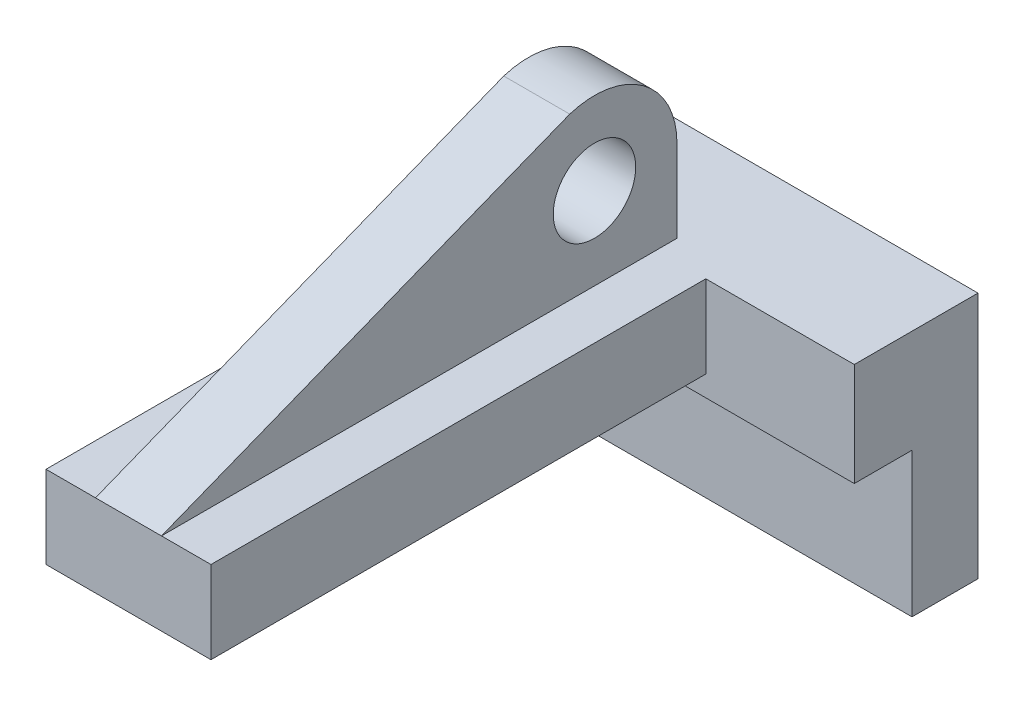
ISO-10303-21;
HEADER;
FILE_DESCRIPTION(('STEP AP214'),'2;1');
FILE_NAME('part.step','',(''),(''),'','','');
FILE_SCHEMA(('AUTOMOTIVE_DESIGN { 1 0 10303 214 1 1 1 1 }'));
ENDSEC;
DATA;
#1=APPLICATION_CONTEXT('core data for automotive mechanical design processes');
#2=APPLICATION_PROTOCOL_DEFINITION('international standard','automotive_design',2000,#1);
#3=PRODUCT_CONTEXT('',#1,'mechanical');
#4=PRODUCT('Part','Part','',(#3));
#5=PRODUCT_RELATED_PRODUCT_CATEGORY('part','',(#4));
#6=PRODUCT_DEFINITION_FORMATION('','',#4);
#7=PRODUCT_DEFINITION_CONTEXT('part definition',#1,'design');
#8=PRODUCT_DEFINITION('design','',#6,#7);
#9=PRODUCT_DEFINITION_SHAPE('','',#8);
#10=(LENGTH_UNIT() NAMED_UNIT(*) SI_UNIT(.MILLI.,.METRE.));
#11=(NAMED_UNIT(*) PLANE_ANGLE_UNIT() SI_UNIT($,.RADIAN.));
#12=(NAMED_UNIT(*) SI_UNIT($,.STERADIAN.) SOLID_ANGLE_UNIT());
#13=UNCERTAINTY_MEASURE_WITH_UNIT(LENGTH_MEASURE(1.E-05),#10,'distance_accuracy_value','');
#14=(GEOMETRIC_REPRESENTATION_CONTEXT(3) GLOBAL_UNCERTAINTY_ASSIGNED_CONTEXT((#13)) GLOBAL_UNIT_ASSIGNED_CONTEXT((#10,
#11,#12)) REPRESENTATION_CONTEXT('',''));
#15=CARTESIAN_POINT('',(0.,0.,0.));
#16=DIRECTION('',(0.,0.,1.));
#17=DIRECTION('',(1.,0.,0.));
#18=AXIS2_PLACEMENT_3D('',#15,#16,#17);
#19=CARTESIAN_POINT('',(0.,0.,25.));
#20=DIRECTION('',(0.,0.,1.));
#21=DIRECTION('',(1.,0.,0.));
#22=AXIS2_PLACEMENT_3D('',#19,#20,#21);
#23=PLANE('',#22);
#24=DIRECTION('',(0.,-1.,0.));
#25=VECTOR('',#24,1.);
#26=CARTESIAN_POINT('',(12.,0.,25.));
#27=LINE('',#26,#25);
#28=CARTESIAN_POINT('',(12.,80.,25.));
#29=VERTEX_POINT('',#28);
#30=CARTESIAN_POINT('',(12.,60.,25.));
#31=VERTEX_POINT('',#30);
#32=EDGE_CURVE('E158',#29,#31,#27,.T.);
#33=ORIENTED_EDGE('',*,*,#32,.F.);
#34=DIRECTION('',(1.,0.,0.));
#35=VECTOR('',#34,1.);
#36=CARTESIAN_POINT('',(0.,80.,25.));
#37=LINE('',#36,#35);
#38=CARTESIAN_POINT('',(28.,80.,25.));
#39=VERTEX_POINT('',#38);
#40=EDGE_CURVE('E61',#29,#39,#37,.T.);
#41=ORIENTED_EDGE('',*,*,#40,.T.);
#42=DIRECTION('',(0.,1.,0.));
#43=VECTOR('',#42,1.);
#44=CARTESIAN_POINT('',(28.,0.,25.));
#45=LINE('',#44,#43);
#46=CARTESIAN_POINT('',(28.,60.,25.));
#47=VERTEX_POINT('',#46);
#48=EDGE_CURVE('E161',#47,#39,#45,.T.);
#49=ORIENTED_EDGE('',*,*,#48,.F.);
#50=DIRECTION('',(1.,0.,0.));
#51=VECTOR('',#50,1.);
#52=CARTESIAN_POINT('',(0.,60.,25.));
#53=LINE('',#52,#51);
#54=EDGE_CURVE('E146',#31,#47,#53,.T.);
#55=ORIENTED_EDGE('',*,*,#54,.F.);
#56=EDGE_LOOP('',(#33,#41,#49,#55));
#57=FACE_BOUND('',#56,.T.);
#58=ADVANCED_FACE('F47',(#57),#23,.F.);
#59=CARTESIAN_POINT('',(0.,103.13948453494,40.7127457797623));
#60=DIRECTION('',(0.,-0.930155863944916,-0.367164906777439));
#61=DIRECTION('',(0.,0.367164906777439,-0.930155863944917));
#62=AXIS2_PLACEMENT_3D('',#59,#60,#61);
#63=PLANE('',#62);
#64=DIRECTION('',(0.,0.367164906777439,-0.930155863944917));
#65=VECTOR('',#64,1.);
#66=CARTESIAN_POINT('',(12.,103.13948453494,40.7127457797623));
#67=LINE('',#66,#65);
#68=CARTESIAN_POINT('',(12.,60.,150.));
#69=VERTEX_POINT('',#68);
#70=CARTESIAN_POINT('',(12.,99.0789287138878,50.9995399098919));
#71=VERTEX_POINT('',#70);
#72=EDGE_CURVE('E155',#69,#71,#67,.T.);
#73=ORIENTED_EDGE('',*,*,#72,.F.);
#74=DIRECTION('',(-1.,0.,0.));
#75=VECTOR('',#74,1.);
#76=CARTESIAN_POINT('',(40.,60.,150.));
#77=LINE('',#76,#75);
#78=CARTESIAN_POINT('',(28.,60.,150.));
#79=VERTEX_POINT('',#78);
#80=EDGE_CURVE('E192',#79,#69,#77,.T.);
#81=ORIENTED_EDGE('',*,*,#80,.F.);
#82=DIRECTION('',(0.,-0.367164906777439,0.930155863944917));
#83=VECTOR('',#82,1.);
#84=CARTESIAN_POINT('',(28.,103.13948453494,40.7127457797623));
#85=LINE('',#84,#83);
#86=CARTESIAN_POINT('',(28.,99.0789287138879,50.9995399098919));
#87=VERTEX_POINT('',#86);
#88=EDGE_CURVE('E523',#87,#79,#85,.T.);
#89=ORIENTED_EDGE('',*,*,#88,.F.);
#90=DIRECTION('',(1.,0.,0.));
#91=VECTOR('',#90,1.);
#92=CARTESIAN_POINT('',(0.,99.0789287138878,50.9995399098919));
#93=LINE('',#92,#91);
#94=EDGE_CURVE('E165',#71,#87,#93,.T.);
#95=ORIENTED_EDGE('',*,*,#94,.F.);
#96=EDGE_LOOP('',(#73,#81,#89,#95));
#97=FACE_BOUND('',#96,.T.);
#98=ADVANCED_FACE('F270',(#97),#63,.F.);
#99=CARTESIAN_POINT('',(0.,80.,45.));
#100=DIRECTION('',(1.,0.,0.));
#101=DIRECTION('',(0.,0.,-1.));
#102=AXIS2_PLACEMENT_3D('',#99,#100,#101);
#103=CYLINDRICAL_SURFACE('',#102,20.);
#104=ORIENTED_EDGE('',*,*,#40,.F.);
#105=CARTESIAN_POINT('',(12.,80.,45.));
#106=DIRECTION('',(-1.,0.,0.));
#107=DIRECTION('',(0.,0.,1.));
#108=AXIS2_PLACEMENT_3D('',#105,#106,#107);
#109=CIRCLE('',#108,20.);
#110=EDGE_CURVE('E156',#71,#29,#109,.T.);
#111=ORIENTED_EDGE('',*,*,#110,.F.);
#112=ORIENTED_EDGE('',*,*,#94,.T.);
#113=CARTESIAN_POINT('',(28.,80.,45.));
#114=DIRECTION('',(1.,0.,0.));
#115=DIRECTION('',(0.,0.,-1.));
#116=AXIS2_PLACEMENT_3D('',#113,#114,#115);
#117=CIRCLE('',#116,20.);
#118=EDGE_CURVE('E172',#39,#87,#117,.T.);
#119=ORIENTED_EDGE('',*,*,#118,.F.);
#120=EDGE_LOOP('',(#104,#111,#112,#119));
#121=FACE_BOUND('',#120,.T.);
#122=ADVANCED_FACE('F269',(#121),#103,.T.);
#123=CARTESIAN_POINT('',(0.,60.,16.));
#124=DIRECTION('',(1.,0.,0.));
#125=DIRECTION('',(0.,0.,-1.));
#126=AXIS2_PLACEMENT_3D('',#123,#124,#125);
#127=PLANE('',#126);
#128=DIRECTION('',(0.,1.,0.));
#129=VECTOR('',#128,1.);
#130=CARTESIAN_POINT('',(0.,60.,150.));
#131=LINE('',#130,#129);
#132=CARTESIAN_POINT('',(0.,40.,150.));
#133=VERTEX_POINT('',#132);
#134=CARTESIAN_POINT('',(0.,60.,150.));
#135=VERTEX_POINT('',#134);
#136=EDGE_CURVE('E168',#133,#135,#131,.T.);
#137=ORIENTED_EDGE('',*,*,#136,.T.);
#138=DIRECTION('',(0.,0.,-1.));
#139=VECTOR('',#138,1.);
#140=CARTESIAN_POINT('',(0.,60.,16.));
#141=LINE('',#140,#139);
#142=CARTESIAN_POINT('',(0.,60.,0.));
#143=VERTEX_POINT('',#142);
#144=EDGE_CURVE('E218',#135,#143,#141,.T.);
#145=ORIENTED_EDGE('',*,*,#144,.T.);
#146=DIRECTION('',(0.,-1.,0.));
#147=VECTOR('',#146,1.);
#148=CARTESIAN_POINT('',(0.,60.,0.));
#149=LINE('',#148,#147);
#150=CARTESIAN_POINT('',(0.,0.,0.));
#151=VERTEX_POINT('',#150);
#152=EDGE_CURVE('E208',#143,#151,#149,.T.);
#153=ORIENTED_EDGE('',*,*,#152,.T.);
#154=DIRECTION('',(0.,0.,-1.));
#155=VECTOR('',#154,1.);
#156=CARTESIAN_POINT('',(0.,0.,16.));
#157=LINE('',#156,#155);
#158=CARTESIAN_POINT('',(0.,0.,16.));
#159=VERTEX_POINT('',#158);
#160=EDGE_CURVE('E12',#159,#151,#157,.T.);
#161=ORIENTED_EDGE('',*,*,#160,.F.);
#162=DIRECTION('',(0.,-1.,0.));
#163=VECTOR('',#162,1.);
#164=CARTESIAN_POINT('',(0.,60.,16.));
#165=LINE('',#164,#163);
#166=CARTESIAN_POINT('',(0.,35.,16.));
#167=VERTEX_POINT('',#166);
#168=EDGE_CURVE('E212',#167,#159,#165,.T.);
#169=ORIENTED_EDGE('',*,*,#168,.F.);
#170=DIRECTION('',(0.,0.,-1.));
#171=VECTOR('',#170,1.);
#172=CARTESIAN_POINT('',(0.,35.,46.));
#173=LINE('',#172,#171);
#174=CARTESIAN_POINT('',(0.,35.,30.));
#175=VERTEX_POINT('',#174);
#176=EDGE_CURVE('E205',#175,#167,#173,.T.);
#177=ORIENTED_EDGE('',*,*,#176,.F.);
#178=DIRECTION('',(0.,-1.,0.));
#179=VECTOR('',#178,1.);
#180=CARTESIAN_POINT('',(0.,35.,30.));
#181=LINE('',#180,#179);
#182=CARTESIAN_POINT('',(0.,40.,30.));
#183=VERTEX_POINT('',#182);
#184=EDGE_CURVE('E188',#183,#175,#181,.T.);
#185=ORIENTED_EDGE('',*,*,#184,.F.);
#186=DIRECTION('',(0.,0.,1.));
#187=VECTOR('',#186,1.);
#188=CARTESIAN_POINT('',(0.,40.,150.));
#189=LINE('',#188,#187);
#190=EDGE_CURVE('E74',#183,#133,#189,.T.);
#191=ORIENTED_EDGE('',*,*,#190,.T.);
#192=EDGE_LOOP('',(#137,#145,#153,#161,#169,#177,#185,#191));
#193=FACE_BOUND('',#192,.T.);
#194=ADVANCED_FACE('F51',(#193),#127,.F.);
#195=CARTESIAN_POINT('',(0.,0.,16.));
#196=DIRECTION('',(0.,1.,0.));
#197=DIRECTION('',(0.,0.,1.));
#198=AXIS2_PLACEMENT_3D('',#195,#196,#197);
#199=PLANE('',#198);
#200=DIRECTION('',(1.,0.,0.));
#201=VECTOR('',#200,1.);
#202=CARTESIAN_POINT('',(0.,0.,0.));
#203=LINE('',#202,#201);
#204=CARTESIAN_POINT('',(76.,0.,0.));
#205=VERTEX_POINT('',#204);
#206=EDGE_CURVE('E224',#151,#205,#203,.T.);
#207=ORIENTED_EDGE('',*,*,#206,.T.);
#208=DIRECTION('',(0.,0.,-1.));
#209=VECTOR('',#208,1.);
#210=CARTESIAN_POINT('',(76.,0.,16.));
#211=LINE('',#210,#209);
#212=CARTESIAN_POINT('',(76.,0.,16.));
#213=VERTEX_POINT('',#212);
#214=EDGE_CURVE('E60',#213,#205,#211,.T.);
#215=ORIENTED_EDGE('',*,*,#214,.F.);
#216=DIRECTION('',(1.,0.,0.));
#217=VECTOR('',#216,1.);
#218=CARTESIAN_POINT('',(0.,0.,16.));
#219=LINE('',#218,#217);
#220=EDGE_CURVE('E214',#159,#213,#219,.T.);
#221=ORIENTED_EDGE('',*,*,#220,.F.);
#222=ORIENTED_EDGE('',*,*,#160,.T.);
#223=EDGE_LOOP('',(#207,#215,#221,#222));
#224=FACE_BOUND('',#223,.T.);
#225=ADVANCED_FACE('F256',(#224),#199,.F.);
#226=CARTESIAN_POINT('',(76.,0.,16.));
#227=DIRECTION('',(-1.,0.,0.));
#228=DIRECTION('',(0.,0.,1.));
#229=AXIS2_PLACEMENT_3D('',#226,#227,#228);
#230=PLANE('',#229);
#231=DIRECTION('',(0.,0.,-1.));
#232=VECTOR('',#231,1.);
#233=CARTESIAN_POINT('',(76.,60.,16.));
#234=LINE('',#233,#232);
#235=CARTESIAN_POINT('',(76.,60.,30.));
#236=VERTEX_POINT('',#235);
#237=CARTESIAN_POINT('',(76.,60.,0.));
#238=VERTEX_POINT('',#237);
#239=EDGE_CURVE('E229',#236,#238,#234,.T.);
#240=ORIENTED_EDGE('',*,*,#239,.F.);
#241=DIRECTION('',(0.,1.,0.));
#242=VECTOR('',#241,1.);
#243=CARTESIAN_POINT('',(76.,60.,30.));
#244=LINE('',#243,#242);
#245=CARTESIAN_POINT('',(76.,35.,30.));
#246=VERTEX_POINT('',#245);
#247=EDGE_CURVE('E199',#246,#236,#244,.T.);
#248=ORIENTED_EDGE('',*,*,#247,.F.);
#249=DIRECTION('',(0.,0.,-1.));
#250=VECTOR('',#249,1.);
#251=CARTESIAN_POINT('',(76.,35.,46.));
#252=LINE('',#251,#250);
#253=CARTESIAN_POINT('',(76.,35.,16.));
#254=VERTEX_POINT('',#253);
#255=EDGE_CURVE('E202',#246,#254,#252,.T.);
#256=ORIENTED_EDGE('',*,*,#255,.T.);
#257=DIRECTION('',(0.,1.,0.));
#258=VECTOR('',#257,1.);
#259=CARTESIAN_POINT('',(76.,0.,16.));
#260=LINE('',#259,#258);
#261=EDGE_CURVE('E216',#213,#254,#260,.T.);
#262=ORIENTED_EDGE('',*,*,#261,.F.);
#263=ORIENTED_EDGE('',*,*,#214,.T.);
#264=DIRECTION('',(0.,1.,0.));
#265=VECTOR('',#264,1.);
#266=CARTESIAN_POINT('',(76.,0.,0.));
#267=LINE('',#266,#265);
#268=EDGE_CURVE('E225',#205,#238,#267,.T.);
#269=ORIENTED_EDGE('',*,*,#268,.T.);
#270=EDGE_LOOP('',(#240,#248,#256,#262,#263,#269));
#271=FACE_BOUND('',#270,.T.);
#272=ADVANCED_FACE('F240',(#271),#230,.F.);
#273=CARTESIAN_POINT('',(76.,60.,16.));
#274=DIRECTION('',(0.,-1.,0.));
#275=DIRECTION('',(0.,0.,-1.));
#276=AXIS2_PLACEMENT_3D('',#273,#274,#275);
#277=PLANE('',#276);
#278=DIRECTION('',(0.,0.,-1.));
#279=VECTOR('',#278,1.);
#280=CARTESIAN_POINT('',(40.,60.,0.));
#281=LINE('',#280,#279);
#282=CARTESIAN_POINT('',(40.,60.,150.));
#283=VERTEX_POINT('',#282);
#284=CARTESIAN_POINT('',(40.,60.,30.));
#285=VERTEX_POINT('',#284);
#286=EDGE_CURVE('E167',#283,#285,#281,.T.);
#287=ORIENTED_EDGE('',*,*,#286,.T.);
#288=DIRECTION('',(-1.,0.,0.));
#289=VECTOR('',#288,1.);
#290=CARTESIAN_POINT('',(0.,60.,30.));
#291=LINE('',#290,#289);
#292=EDGE_CURVE('E200',#236,#285,#291,.T.);
#293=ORIENTED_EDGE('',*,*,#292,.F.);
#294=ORIENTED_EDGE('',*,*,#239,.T.);
#295=DIRECTION('',(-1.,0.,0.));
#296=VECTOR('',#295,1.);
#297=CARTESIAN_POINT('',(76.,60.,0.));
#298=LINE('',#297,#296);
#299=EDGE_CURVE('E211',#238,#143,#298,.T.);
#300=ORIENTED_EDGE('',*,*,#299,.T.);
#301=ORIENTED_EDGE('',*,*,#144,.F.);
#302=DIRECTION('',(-1.,0.,0.));
#303=VECTOR('',#302,1.);
#304=CARTESIAN_POINT('',(12.,60.,150.));
#305=LINE('',#304,#303);
#306=EDGE_CURVE('E152',#69,#135,#305,.T.);
#307=ORIENTED_EDGE('',*,*,#306,.F.);
#308=DIRECTION('',(0.,0.,1.));
#309=VECTOR('',#308,1.);
#310=CARTESIAN_POINT('',(12.,60.,0.));
#311=LINE('',#310,#309);
#312=EDGE_CURVE('E143',#31,#69,#311,.T.);
#313=ORIENTED_EDGE('',*,*,#312,.F.);
#314=ORIENTED_EDGE('',*,*,#54,.T.);
#315=DIRECTION('',(0.,0.,-1.));
#316=VECTOR('',#315,1.);
#317=CARTESIAN_POINT('',(28.,60.,0.));
#318=LINE('',#317,#316);
#319=EDGE_CURVE('E518',#79,#47,#318,.T.);
#320=ORIENTED_EDGE('',*,*,#319,.F.);
#321=EDGE_CURVE('E190',#283,#79,#77,.T.);
#322=ORIENTED_EDGE('',*,*,#321,.F.);
#323=EDGE_LOOP('',(#287,#293,#294,#300,#301,#307,#313,#314,#320,#322));
#324=FACE_BOUND('',#323,.T.);
#325=ADVANCED_FACE('F150',(#324),#277,.F.);
#326=CARTESIAN_POINT('',(0.,0.,16.));
#327=DIRECTION('',(0.,0.,1.));
#328=DIRECTION('',(1.,0.,0.));
#329=AXIS2_PLACEMENT_3D('',#326,#327,#328);
#330=PLANE('',#329);
#331=DIRECTION('',(1.,0.,0.));
#332=VECTOR('',#331,1.);
#333=CARTESIAN_POINT('',(0.,35.,16.));
#334=LINE('',#333,#332);
#335=EDGE_CURVE('E207',#167,#254,#334,.T.);
#336=ORIENTED_EDGE('',*,*,#335,.F.);
#337=ORIENTED_EDGE('',*,*,#168,.T.);
#338=ORIENTED_EDGE('',*,*,#220,.T.);
#339=ORIENTED_EDGE('',*,*,#261,.T.);
#340=EDGE_LOOP('',(#336,#337,#338,#339));
#341=FACE_BOUND('',#340,.T.);
#342=ADVANCED_FACE('F253',(#341),#330,.T.);
#343=CARTESIAN_POINT('',(0.,0.,0.));
#344=DIRECTION('',(0.,0.,1.));
#345=DIRECTION('',(1.,0.,0.));
#346=AXIS2_PLACEMENT_3D('',#343,#344,#345);
#347=PLANE('',#346);
#348=ORIENTED_EDGE('',*,*,#152,.F.);
#349=ORIENTED_EDGE('',*,*,#299,.F.);
#350=ORIENTED_EDGE('',*,*,#268,.F.);
#351=ORIENTED_EDGE('',*,*,#206,.F.);
#352=EDGE_LOOP('',(#348,#349,#350,#351));
#353=FACE_BOUND('',#352,.T.);
#354=ADVANCED_FACE('F243',(#353),#347,.F.);
#355=CARTESIAN_POINT('',(0.,35.,46.));
#356=DIRECTION('',(0.,-1.,0.));
#357=DIRECTION('',(0.,0.,-1.));
#358=AXIS2_PLACEMENT_3D('',#355,#356,#357);
#359=PLANE('',#358);
#360=DIRECTION('',(1.,0.,0.));
#361=VECTOR('',#360,1.);
#362=CARTESIAN_POINT('',(76.,35.,30.));
#363=LINE('',#362,#361);
#364=EDGE_CURVE('E196',#175,#246,#363,.T.);
#365=ORIENTED_EDGE('',*,*,#364,.F.);
#366=ORIENTED_EDGE('',*,*,#176,.T.);
#367=ORIENTED_EDGE('',*,*,#335,.T.);
#368=ORIENTED_EDGE('',*,*,#255,.F.);
#369=EDGE_LOOP('',(#365,#366,#367,#368));
#370=FACE_BOUND('',#369,.T.);
#371=ADVANCED_FACE('F249',(#370),#359,.T.);
#372=CARTESIAN_POINT('',(0.,0.,30.));
#373=DIRECTION('',(0.,0.,-1.));
#374=DIRECTION('',(-1.,0.,0.));
#375=AXIS2_PLACEMENT_3D('',#372,#373,#374);
#376=PLANE('',#375);
#377=ORIENTED_EDGE('',*,*,#292,.T.);
#378=DIRECTION('',(0.,-1.,0.));
#379=VECTOR('',#378,1.);
#380=CARTESIAN_POINT('',(40.,40.,30.));
#381=LINE('',#380,#379);
#382=CARTESIAN_POINT('',(40.,40.,30.));
#383=VERTEX_POINT('',#382);
#384=EDGE_CURVE('E174',#285,#383,#381,.T.);
#385=ORIENTED_EDGE('',*,*,#384,.T.);
#386=DIRECTION('',(-1.,0.,0.));
#387=VECTOR('',#386,1.);
#388=CARTESIAN_POINT('',(40.,40.,30.));
#389=LINE('',#388,#387);
#390=EDGE_CURVE('E182',#383,#183,#389,.T.);
#391=ORIENTED_EDGE('',*,*,#390,.T.);
#392=ORIENTED_EDGE('',*,*,#184,.T.);
#393=ORIENTED_EDGE('',*,*,#364,.T.);
#394=ORIENTED_EDGE('',*,*,#247,.T.);
#395=EDGE_LOOP('',(#377,#385,#391,#392,#393,#394));
#396=FACE_BOUND('',#395,.T.);
#397=ADVANCED_FACE('F289',(#396),#376,.F.);
#398=CARTESIAN_POINT('',(40.,60.,150.));
#399=DIRECTION('',(0.,0.,1.));
#400=DIRECTION('',(1.,0.,0.));
#401=AXIS2_PLACEMENT_3D('',#398,#399,#400);
#402=PLANE('',#401);
#403=ORIENTED_EDGE('',*,*,#136,.F.);
#404=DIRECTION('',(-1.,0.,0.));
#405=VECTOR('',#404,1.);
#406=CARTESIAN_POINT('',(40.,40.,150.));
#407=LINE('',#406,#405);
#408=CARTESIAN_POINT('',(40.,40.,150.));
#409=VERTEX_POINT('',#408);
#410=EDGE_CURVE('E195',#409,#133,#407,.T.);
#411=ORIENTED_EDGE('',*,*,#410,.F.);
#412=DIRECTION('',(0.,1.,0.));
#413=VECTOR('',#412,1.);
#414=CARTESIAN_POINT('',(40.,60.,150.));
#415=LINE('',#414,#413);
#416=EDGE_CURVE('E181',#409,#283,#415,.T.);
#417=ORIENTED_EDGE('',*,*,#416,.T.);
#418=ORIENTED_EDGE('',*,*,#321,.T.);
#419=ORIENTED_EDGE('',*,*,#80,.T.);
#420=ORIENTED_EDGE('',*,*,#306,.T.);
#421=EDGE_LOOP('',(#403,#411,#417,#418,#419,#420));
#422=FACE_BOUND('',#421,.T.);
#423=ADVANCED_FACE('F283',(#422),#402,.T.);
#424=CARTESIAN_POINT('',(40.,40.,150.));
#425=DIRECTION('',(0.,-1.,0.));
#426=DIRECTION('',(0.,0.,-1.));
#427=AXIS2_PLACEMENT_3D('',#424,#425,#426);
#428=PLANE('',#427);
#429=ORIENTED_EDGE('',*,*,#190,.F.);
#430=ORIENTED_EDGE('',*,*,#390,.F.);
#431=DIRECTION('',(0.,0.,1.));
#432=VECTOR('',#431,1.);
#433=CARTESIAN_POINT('',(40.,40.,150.));
#434=LINE('',#433,#432);
#435=EDGE_CURVE('E178',#383,#409,#434,.T.);
#436=ORIENTED_EDGE('',*,*,#435,.T.);
#437=ORIENTED_EDGE('',*,*,#410,.T.);
#438=EDGE_LOOP('',(#429,#430,#436,#437));
#439=FACE_BOUND('',#438,.T.);
#440=ADVANCED_FACE('F282',(#439),#428,.T.);
#441=CARTESIAN_POINT('',(40.,0.,0.));
#442=DIRECTION('',(1.,0.,0.));
#443=DIRECTION('',(0.,0.,-1.));
#444=AXIS2_PLACEMENT_3D('',#441,#442,#443);
#445=PLANE('',#444);
#446=ORIENTED_EDGE('',*,*,#286,.F.);
#447=ORIENTED_EDGE('',*,*,#416,.F.);
#448=ORIENTED_EDGE('',*,*,#435,.F.);
#449=ORIENTED_EDGE('',*,*,#384,.F.);
#450=EDGE_LOOP('',(#446,#447,#448,#449));
#451=FACE_BOUND('',#450,.T.);
#452=ADVANCED_FACE('F279',(#451),#445,.T.);
#453=CARTESIAN_POINT('',(28.,0.,0.));
#454=DIRECTION('',(1.,0.,0.));
#455=DIRECTION('',(0.,0.,-1.));
#456=AXIS2_PLACEMENT_3D('',#453,#454,#455);
#457=PLANE('',#456);
#458=CARTESIAN_POINT('',(28.,80.,45.));
#459=DIRECTION('',(1.,0.,0.));
#460=DIRECTION('',(0.,0.,-1.));
#461=AXIS2_PLACEMENT_3D('',#458,#459,#460);
#462=CIRCLE('',#461,10.);
#463=CARTESIAN_POINT('',(28.,80.,35.));
#464=VERTEX_POINT('',#463);
#465=EDGE_CURVE('E530',#464,#464,#462,.T.);
#466=ORIENTED_EDGE('',*,*,#465,.F.);
#467=EDGE_LOOP('',(#466));
#468=FACE_BOUND('',#467,.T.);
#469=ORIENTED_EDGE('',*,*,#88,.T.);
#470=ORIENTED_EDGE('',*,*,#319,.T.);
#471=ORIENTED_EDGE('',*,*,#48,.T.);
#472=ORIENTED_EDGE('',*,*,#118,.T.);
#473=EDGE_LOOP('',(#469,#470,#471,#472));
#474=FACE_BOUND('',#473,.T.);
#475=ADVANCED_FACE('F281',(#468,#474),#457,.T.);
#476=CARTESIAN_POINT('',(12.,0.,0.));
#477=DIRECTION('',(-1.,0.,0.));
#478=DIRECTION('',(0.,0.,1.));
#479=AXIS2_PLACEMENT_3D('',#476,#477,#478);
#480=PLANE('',#479);
#481=CARTESIAN_POINT('',(12.,80.,45.));
#482=DIRECTION('',(1.,0.,0.));
#483=DIRECTION('',(0.,0.,-1.));
#484=AXIS2_PLACEMENT_3D('',#481,#482,#483);
#485=CIRCLE('',#484,10.);
#486=CARTESIAN_POINT('',(12.,80.,35.));
#487=VERTEX_POINT('',#486);
#488=EDGE_CURVE('E163',#487,#487,#485,.T.);
#489=ORIENTED_EDGE('',*,*,#488,.T.);
#490=EDGE_LOOP('',(#489));
#491=FACE_BOUND('',#490,.T.);
#492=ORIENTED_EDGE('',*,*,#32,.T.);
#493=ORIENTED_EDGE('',*,*,#312,.T.);
#494=ORIENTED_EDGE('',*,*,#72,.T.);
#495=ORIENTED_EDGE('',*,*,#110,.T.);
#496=EDGE_LOOP('',(#492,#493,#494,#495));
#497=FACE_BOUND('',#496,.T.);
#498=ADVANCED_FACE('F157',(#491,#497),#480,.T.);
#499=CARTESIAN_POINT('',(12.,80.,45.));
#500=DIRECTION('',(1.,0.,0.));
#501=DIRECTION('',(0.,0.,-1.));
#502=AXIS2_PLACEMENT_3D('',#499,#500,#501);
#503=CYLINDRICAL_SURFACE('',#502,10.);
#504=ORIENTED_EDGE('',*,*,#488,.F.);
#505=EDGE_LOOP('',(#504));
#506=FACE_BOUND('',#505,.T.);
#507=ORIENTED_EDGE('',*,*,#465,.T.);
#508=EDGE_LOOP('',(#507));
#509=FACE_BOUND('',#508,.T.);
#510=ADVANCED_FACE('F339',(#506,#509),#503,.F.);
#511=CLOSED_SHELL('',(#58,#98,#122,#194,#225,#272,#325,#342,#354,#371,#397,#423,#440,#452,#475,
#498,#510));
#512=MANIFOLD_SOLID_BREP('B2',#511);
#513=ADVANCED_BREP_SHAPE_REPRESENTATION('',(#18,#512),#14);
#514=SHAPE_DEFINITION_REPRESENTATION(#9,#513);
ENDSEC;
END-ISO-10303-21;
